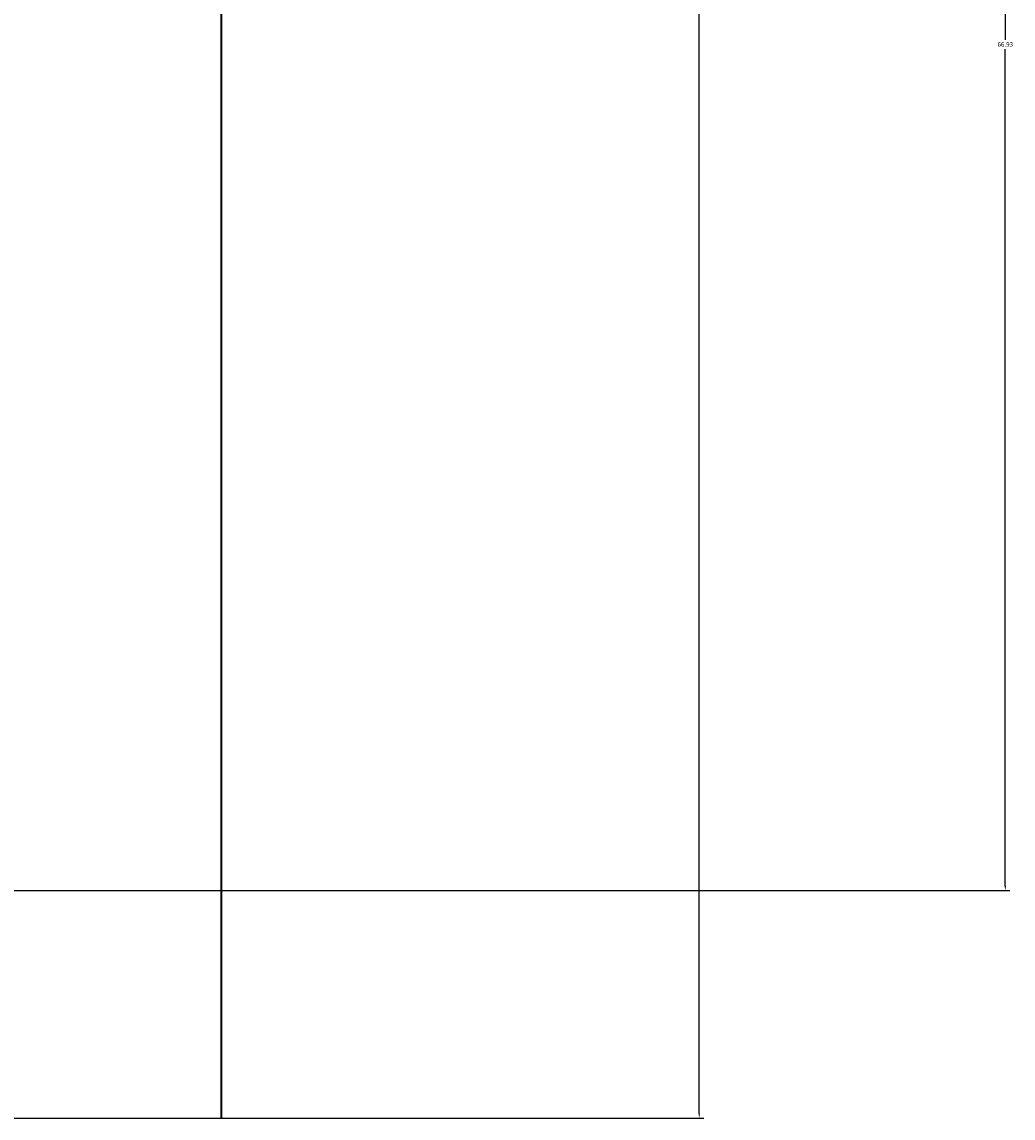
# Model space of a CAD drawing. Units: feet. Extents: x 1654 to 2985, y 1348 to 2230.
# Tile 21 of 53: x 2203 to 2242, y 1565 to 1609. Entities that reach past the tile are written whole.
import ezdxf

# ---------------------------------------------------------------- set-up
doc = ezdxf.new("R2010")
doc.units = ezdxf.units.FT
for name, color, linetype, lineweight in [('A-ANNO-DIMS', 2, 'Continuous', 18), ('A-FLOR', 7, 'Continuous', 25), ('A-WALL', 7, 'Continuous', 35)]:
    doc.layers.add(name, color=color, linetype=linetype, lineweight=lineweight)
doc.styles.get("Standard").update_dxf_attribs({"font": 'arial.ttf'})
doc.dimstyles.get("Standard").update_dxf_attribs({"dimtxt": 0.18, "dimasz": 0.18, "dimexe": 0.18, "dimexo": 0.0625, "dimgap": 0.09, "dimtad": 0, "dimtih": 1, "dimtoh": 1, "dimdec": 4, "dimzin": 0, "dimdsep": 46, "dimtxsty": 'Standard', "dimcen": 0.09, "dimadec": 0, "dimazin": 0, "dimtfac": 1, "dimtdec": 4, "dimtofl": 0, "dimtmove": 0, "dimatfit": 3, "dimfxl": 1, "dimtolj": 1, "dimtzin": 0, "dimarcsym": 0})

# ---------------------------------------------------------------- blocks, each defined once
blk = doc.blocks.new('*D72')
at = {"layer": 'A-ANNO-DIMS', "color": 0, "lineweight": -2, "transparency": 16777216}
for p, q in [((2202.155, 1751.255), (2230.172, 1751.255)), ((2229.992, 1751.075), (2229.992, 1658.438)), ((2229.992, 1565.435), (2229.992, 1658.072)), ((2202.155, 1565.255), (2230.172, 1565.255))]:
    blk.add_line(p, q, dxfattribs=at)
at = {"layer": 'A-ANNO-DIMS', "color": 0, "transparency": 16777216}
for points in [[(2229.962, 1751.075), (2230.022, 1751.075), (2229.992, 1751.255)], [(2229.962, 1565.435), (2230.022, 1565.435), (2229.992, 1565.255)]]:
    blk.add_solid(points, dxfattribs=at)
at = {"layer": 'Defpoints', "color": 0, "transparency": 16777216}
for p in [(2202.092, 1751.255), (2229.992, 1751.255), (2202.092, 1565.255)]:
    blk.add_point(p, dxfattribs=at)
at = {"layer": 'A-ANNO-DIMS', "color": 0, "transparency": 16777216, "insert": (2229.992, 1658.255), "char_height": 0.18, "attachment_point": 5}
blk.add_mtext('\\A1;STAIR 186 TYP.', dxfattribs=at)
blk = doc.blocks.new('*D90')
at = {"layer": 'A-ANNO-DIMS', "color": 0, "lineweight": -2, "transparency": 16777216}
for p, q in [((1852.155, 1641.187), (2242.272, 1641.187)), ((2242.092, 1641.007), (2242.092, 1607.903)), ((2242.092, 1574.435), (2242.092, 1607.539)), ((1852.155, 1574.255), (2242.272, 1574.255))]:
    blk.add_line(p, q, dxfattribs=at)
at = {"layer": 'A-ANNO-DIMS', "color": 0, "transparency": 16777216}
for points in [[(2242.062, 1641.007), (2242.122, 1641.007), (2242.092, 1641.187)], [(2242.062, 1574.435), (2242.122, 1574.435), (2242.092, 1574.255)]]:
    blk.add_solid(points, dxfattribs=at)
at = {"layer": 'Defpoints', "color": 0, "transparency": 16777216}
for p in [(1852.092, 1641.187), (2242.092, 1641.187), (1852.092, 1574.255)]:
    blk.add_point(p, dxfattribs=at)
at = {"layer": 'A-ANNO-DIMS', "color": 0, "transparency": 16777216, "insert": (2242.092, 1607.721), "char_height": 0.18, "attachment_point": 5}
blk.add_mtext('\\A1;66.93', dxfattribs=at)

msp = doc.modelspace()

# ---------------------------------------------------------------- linework, layer by layer
at = {"layer": 'A-FLOR'}
msp.add_line((2008.0924, 1565.2549), (2211.0924, 1565.2549), dxfattribs=at)
at = {"layer": 'A-WALL'}
msp.add_line((2211.0924, 1886.2549), (2211.0924, 1565.2549), dxfattribs=at)

# ---------------------------------------------------------------- dimensions: what is measured, and where the dimension line sits
at = {"layer": 'A-ANNO-DIMS'}
dim = msp.add_linear_dim(base=(2229.9924, 1751.2549), p1=(2202.0924, 1565.2549), p2=(2202.0924, 1751.2549), angle=90, text='STAIR <> TYP.', dimstyle='Standard', override={"dimdec": 0, "dimlfac": 1, "dimrnd": 0, "dimzin": 0, "dimdsep": 46, "dimlunit": 2}, dxfattribs=at)
dim.commit()
dim.dimension.update_dxf_attribs({"geometry": '*D72', "text_midpoint": (2229.9924, 1658.2549)})
dim = msp.add_linear_dim(base=(2242.0924, 1641.187), p1=(1852.0924, 1574.2549), p2=(1852.0924, 1641.187), angle=90, dimstyle='Standard', override={"dimdec": 2, "dimlfac": 1, "dimrnd": 0, "dimzin": 0, "dimdsep": 46, "dimlunit": 2}, dxfattribs=at)
dim.commit()
dim.dimension.update_dxf_attribs({"geometry": '*D90', "text_midpoint": (2242.0924, 1607.721)})

doc.saveas('drawing.dxf')
